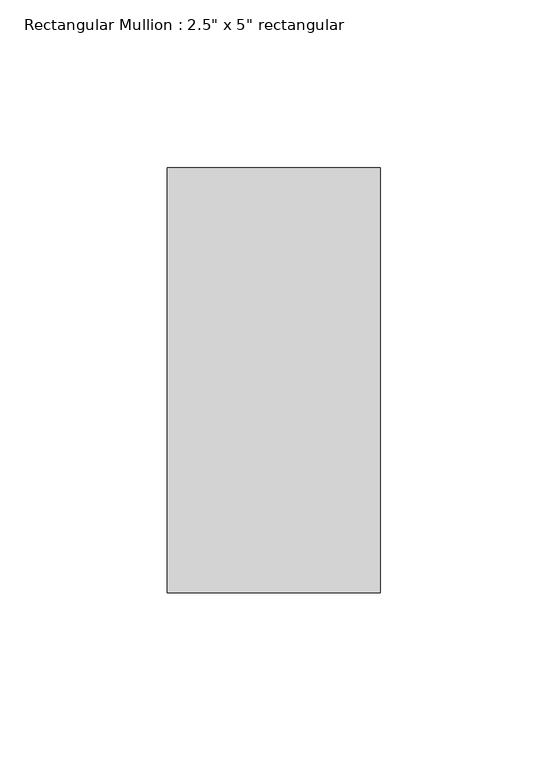
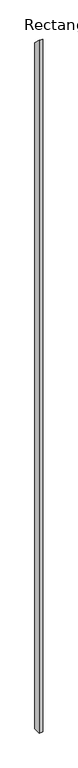
"""IFC4 building model written with IfcOpenShell, lengths in millimetres: member geometry."""

from ifc_helpers import new_model, si_unit, frame, origin, place, context, project, spatial, polyline, outline, extrude, source, transform, mapped, element, save


def member_104e7e8d(model_context):
    return source(origin(), model_context, "Body", "SweptSolid", [
        extrude(outline(polyline([(-63.5, 63.5), (63.5, -63.5), (63.5, -12954.0), (-63.5, -12954.0), (-63.5, 63.5)])), frame((-63.5, 0.0, 0.0), z_axis=(1.0, 0.0, 0.0), x_axis=(0.0, 1.0, 0.0)), (0.0, 0.0, 1.0), 63.5),
    ])


if __name__ == "__main__":
    model = new_model("IFC4")
    model_context = context("Model", 3, world=origin())
    ifc_project = project(units=[si_unit("LENGTHUNIT", "METRE", prefix="MILLI")], contexts=[model_context])
    site = spatial("IfcSite", under=ifc_project)
    building = spatial("IfcBuilding", under=site)
    placement = place(None, origin())
    member_shape = member_104e7e8d(model_context)
    element("IfcMember", 1, ObjectType="Rectangular Mullion : 2.5\" x 5\" rectangular", at=placement, inside=building, context=model_context, shape_type="MappedRepresentation", body=[
        mapped(member_shape, transform((0.0, 0.0, 0.0), x_axis=(1.0, 0.0, 0.0), y_axis=(0.0, 1.0, 0.0), z_axis=(0.0, 0.0, 1.0))),
    ])
    save(model, "model.ifc")

# Revit data of these elements
# Type "Rectangular Mullion : 2.5\" x 5\" rectangular"
#   built-in parameter 1007304 = 0.416667 (stored number, unit not read)
#   built-in parameter 1007301 = 0.104167 (stored number, unit not read)
#   built-in parameter 1007300 = 0.104167 (stored number, unit not read)
# Element 1 (IfcMember, "Rectangular Mullion : 2.5\" x 5\" rectangular")
#   Materials on its faces: "Aluminum"
# Materials
#   "Aluminum": class "Metal", colour RGB 247 247 247, transparency 0, Description = "Aluminum 6061", Cost = 0
